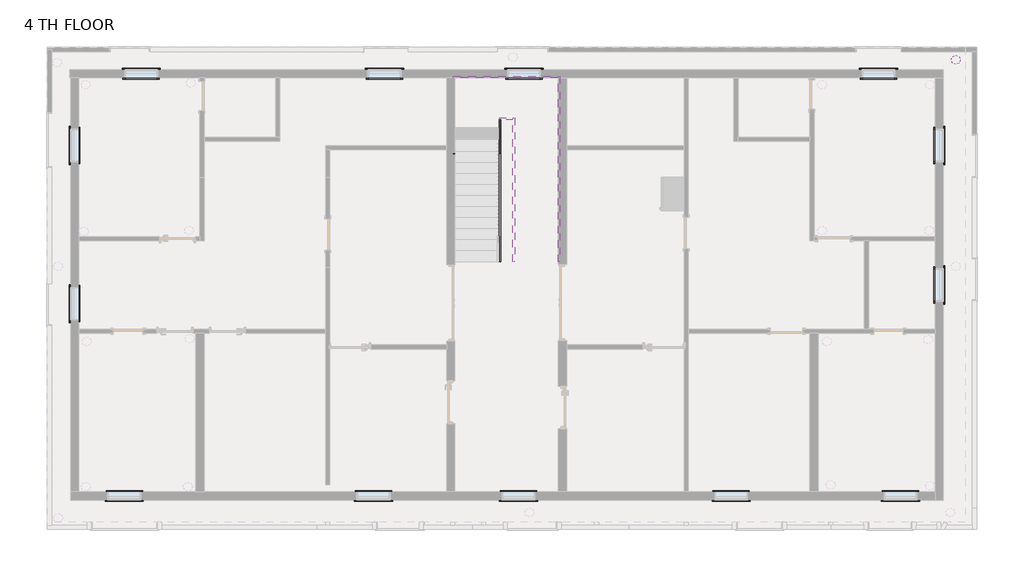
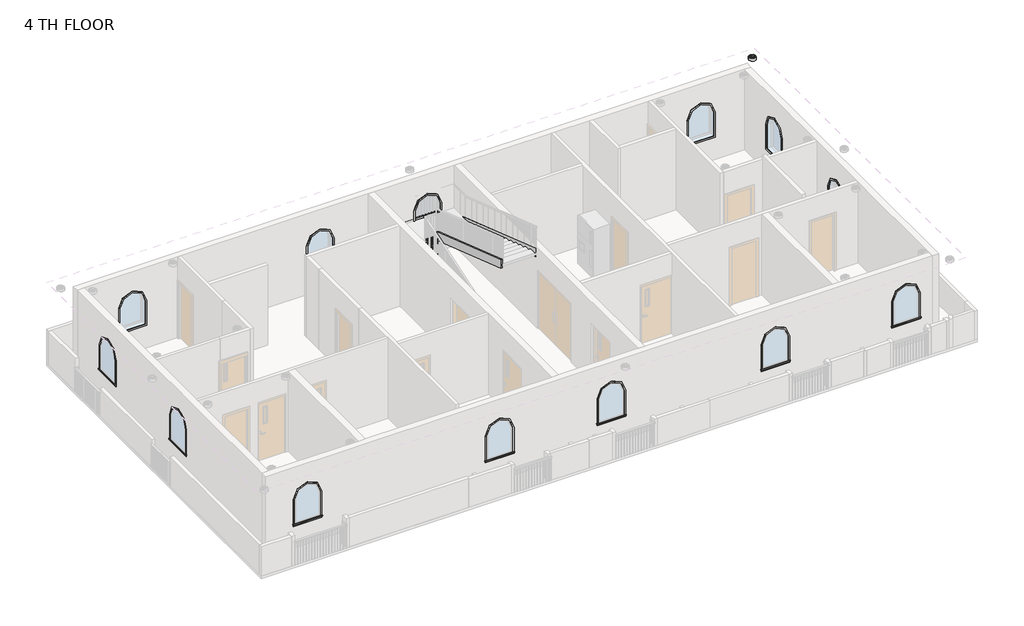
# One storey, part 7 of 7: 26 proxies, 6 members, 1 light fixture.
"""IFC4 building model written with IfcOpenShell, lengths in millimetres."""

from ifc_helpers import new_model, si_unit, frame, origin, place, context, project, spatial, polyline, outline, extrude, transform, mapped, element, save
from components import trim_window_exterior_flat_arch_top_tree_centered_with_sill_aed3e54d, trim_window_interior_flat_arch_top_tree_centered_picture_e2e46177, ceiling_light_flat_round_60w_120v_7c4c2a52

model = new_model("IFC4")

# Units and contexts
model_context = context("Model", 3, world=origin())
ifc_project = project(units=[si_unit("LENGTHUNIT", "METRE", prefix="MILLI")], contexts=[model_context])

# Site, building, storey
site = spatial("IfcSite", under=ifc_project)
building = spatial("IfcBuilding", under=site)
storey = spatial("IfcBuildingStorey", under=building, Name="4 TH FLOOR", Elevation=12801.6)

# Proxies
placement = place(None, origin())
trim_window_exterior_flat_arch_top_tree_centered_with_sill_shape = trim_window_exterior_flat_arch_top_tree_centered_with_sill_aed3e54d(model_context)
element("IfcBuildingElementProxy", 1, Name="Trim-Window-Exterior-Flat-Arch-Top-Tree_Centered : with Sill", ObjectType="Trim-Window-Exterior-Flat-Arch-Top-Tree_Centered : with Sill", at=placement, inside=storey, context=model_context, shape_type="MappedRepresentation", body=[
    mapped(trim_window_exterior_flat_arch_top_tree_centered_with_sill_shape, transform((-10967.3987925, -4014.0932193, 15087.6), x_axis=(1.0, 0.0, 0.0), y_axis=(0.0, 0.0, 1.0), z_axis=(0.0, -1.0, 0.0))),
])
element("IfcBuildingElementProxy", 2, Name="Trim-Window-Exterior-Flat-Arch-Top-Tree_Centered : with Sill", ObjectType="Trim-Window-Exterior-Flat-Arch-Top-Tree_Centered : with Sill", at=placement, inside=storey, context=model_context, shape_type="MappedRepresentation", body=[
    mapped(trim_window_exterior_flat_arch_top_tree_centered_with_sill_shape, transform((-4096.6987998, -4014.0932193, 15087.6), x_axis=(1.0, 0.0, 0.0), y_axis=(0.0, 0.0, 1.0), z_axis=(0.0, -1.0, 0.0))),
])
element("IfcBuildingElementProxy", 3, Name="Trim-Window-Exterior-Flat-Arch-Top-Tree_Centered : with Sill", ObjectType="Trim-Window-Exterior-Flat-Arch-Top-Tree_Centered : with Sill", at=placement, inside=storey, context=model_context, shape_type="MappedRepresentation", body=[
    mapped(trim_window_exterior_flat_arch_top_tree_centered_with_sill_shape, transform((-96.7067989, -4014.0932193, 15087.6), x_axis=(1.0, 0.0, 0.0), y_axis=(0.0, 0.0, 1.0), z_axis=(0.0, -1.0, 0.0))),
])
element("IfcBuildingElementProxy", 4, Name="Trim-Window-Exterior-Flat-Arch-Top-Tree_Centered : with Sill", ObjectType="Trim-Window-Exterior-Flat-Arch-Top-Tree_Centered : with Sill", at=placement, inside=storey, context=model_context, shape_type="MappedRepresentation", body=[
    mapped(trim_window_exterior_flat_arch_top_tree_centered_with_sill_shape, transform((5771.2012079, -4014.0932193, 15087.6), x_axis=(1.0, 0.0, 0.0), y_axis=(0.0, 0.0, 1.0), z_axis=(0.0, -1.0, 0.0))),
])
element("IfcBuildingElementProxy", 5, Name="Trim-Window-Exterior-Flat-Arch-Top-Tree_Centered : with Sill", ObjectType="Trim-Window-Exterior-Flat-Arch-Top-Tree_Centered : with Sill", at=placement, inside=storey, context=model_context, shape_type="MappedRepresentation", body=[
    mapped(trim_window_exterior_flat_arch_top_tree_centered_with_sill_shape, transform((10444.8012075, -4014.0932193, 15087.6), x_axis=(1.0, 0.0, 0.0), y_axis=(0.0, 0.0, 1.0), z_axis=(0.0, -1.0, 0.0))),
])
element("IfcBuildingElementProxy", 6, Name="Trim-Window-Exterior-Flat-Arch-Top-Tree_Centered : with Sill", ObjectType="Trim-Window-Exterior-Flat-Arch-Top-Tree_Centered : with Sill", at=placement, inside=storey, context=model_context, shape_type="MappedRepresentation", body=[
    mapped(trim_window_exterior_flat_arch_top_tree_centered_with_sill_shape, transform((11625.9012075, 1916.8067333, 15087.6), x_axis=(0.0, 1.0, 0.0), y_axis=(0.0, 0.0, 1.0), z_axis=(1.0, 0.0, 0.0))),
])
element("IfcBuildingElementProxy", 7, Name="Trim-Window-Exterior-Flat-Arch-Top-Tree_Centered : with Sill", ObjectType="Trim-Window-Exterior-Flat-Arch-Top-Tree_Centered : with Sill", at=placement, inside=storey, context=model_context, shape_type="MappedRepresentation", body=[
    mapped(trim_window_exterior_flat_arch_top_tree_centered_with_sill_shape, transform((11625.9012075, 5764.9067329, 15087.6), x_axis=(0.0, 1.0, 0.0), y_axis=(0.0, 0.0, 1.0), z_axis=(1.0, 0.0, 0.0))),
])
element("IfcBuildingElementProxy", 8, Name="Trim-Window-Exterior-Flat-Arch-Top-Tree_Centered : with Sill", ObjectType="Trim-Window-Exterior-Flat-Arch-Top-Tree_Centered : with Sill", at=placement, inside=storey, context=model_context, shape_type="MappedRepresentation", body=[
    mapped(trim_window_exterior_flat_arch_top_tree_centered_with_sill_shape, transform((9835.2012075, 7860.4067329, 15087.6), x_axis=(-1.0, 0.0, 0.0), y_axis=(0.0, 0.0, 1.0), z_axis=(0.0, 1.0, 0.0))),
])
element("IfcBuildingElementProxy", 9, Name="Trim-Window-Exterior-Flat-Arch-Top-Tree_Centered : with Sill", ObjectType="Trim-Window-Exterior-Flat-Arch-Top-Tree_Centered : with Sill", at=placement, inside=storey, context=model_context, shape_type="MappedRepresentation", body=[
    mapped(trim_window_exterior_flat_arch_top_tree_centered_with_sill_shape, transform((55.6932011, 7860.4067329, 15087.6), x_axis=(-1.0, 0.0, 0.0), y_axis=(0.0, 0.0, 1.0), z_axis=(0.0, 1.0, 0.0))),
])
element("IfcBuildingElementProxy", 10, Name="Trim-Window-Exterior-Flat-Arch-Top-Tree_Centered : with Sill", ObjectType="Trim-Window-Exterior-Flat-Arch-Top-Tree_Centered : with Sill", at=placement, inside=storey, context=model_context, shape_type="MappedRepresentation", body=[
    mapped(trim_window_exterior_flat_arch_top_tree_centered_with_sill_shape, transform((-3791.8987998, 7860.4067329, 15087.6), x_axis=(-1.0, 0.0, 0.0), y_axis=(0.0, 0.0, 1.0), z_axis=(0.0, 1.0, 0.0))),
])
element("IfcBuildingElementProxy", 11, Name="Trim-Window-Exterior-Flat-Arch-Top-Tree_Centered : with Sill", ObjectType="Trim-Window-Exterior-Flat-Arch-Top-Tree_Centered : with Sill", at=placement, inside=storey, context=model_context, shape_type="MappedRepresentation", body=[
    mapped(trim_window_exterior_flat_arch_top_tree_centered_with_sill_shape, transform((-10503.8487992, 7860.4067329, 15087.6), x_axis=(-1.0, 0.0, 0.0), y_axis=(0.0, 0.0, 1.0), z_axis=(0.0, 1.0, 0.0))),
])
element("IfcBuildingElementProxy", 12, Name="Trim-Window-Exterior-Flat-Arch-Top-Tree_Centered : with Sill", ObjectType="Trim-Window-Exterior-Flat-Arch-Top-Tree_Centered : with Sill", at=placement, inside=storey, context=model_context, shape_type="MappedRepresentation", body=[
    mapped(trim_window_exterior_flat_arch_top_tree_centered_with_sill_shape, transform((-12453.2987925, 5764.9067329, 15087.6), x_axis=(0.0, -1.0, 0.0), y_axis=(0.0, 0.0, 1.0), z_axis=(-1.0, 0.0, 0.0))),
])
element("IfcBuildingElementProxy", 13, Name="Trim-Window-Exterior-Flat-Arch-Top-Tree_Centered : with Sill", ObjectType="Trim-Window-Exterior-Flat-Arch-Top-Tree_Centered : with Sill", at=placement, inside=storey, context=model_context, shape_type="MappedRepresentation", body=[
    mapped(trim_window_exterior_flat_arch_top_tree_centered_with_sill_shape, transform((-12453.2987925, 1402.4567334, 15087.6), x_axis=(0.0, -1.0, 0.0), y_axis=(0.0, 0.0, 1.0), z_axis=(-1.0, 0.0, 0.0))),
])
trim_window_interior_flat_arch_top_tree_centered_picture_shape = trim_window_interior_flat_arch_top_tree_centered_picture_e2e46177(model_context)
element("IfcBuildingElementProxy", 14, Name="Trim-Window-Interior-Flat-Arch-Top-Tree_Centered : Picture Frame", ObjectType="Trim-Window-Interior-Flat-Arch-Top-Tree_Centered : Picture Frame", at=placement, inside=storey, context=model_context, shape_type="MappedRepresentation", body=[
    mapped(trim_window_interior_flat_arch_top_tree_centered_picture_shape, transform((-10967.3987925, -3785.4932193, 15087.6), x_axis=(-1.0, 0.0, 0.0), y_axis=(0.0, 0.0, 1.0), z_axis=(0.0, 1.0, 0.0))),
])
element("IfcBuildingElementProxy", 15, Name="Trim-Window-Interior-Flat-Arch-Top-Tree_Centered : Picture Frame", ObjectType="Trim-Window-Interior-Flat-Arch-Top-Tree_Centered : Picture Frame", at=placement, inside=storey, context=model_context, shape_type="MappedRepresentation", body=[
    mapped(trim_window_interior_flat_arch_top_tree_centered_picture_shape, transform((-4096.6987998, -3785.4932193, 15087.6), x_axis=(-1.0, 0.0, 0.0), y_axis=(0.0, 0.0, 1.0), z_axis=(0.0, 1.0, 0.0))),
])
element("IfcBuildingElementProxy", 16, Name="Trim-Window-Interior-Flat-Arch-Top-Tree_Centered : Picture Frame", ObjectType="Trim-Window-Interior-Flat-Arch-Top-Tree_Centered : Picture Frame", at=placement, inside=storey, context=model_context, shape_type="MappedRepresentation", body=[
    mapped(trim_window_interior_flat_arch_top_tree_centered_picture_shape, transform((-96.7067989, -3785.4932193, 15087.6), x_axis=(-1.0, 0.0, 0.0), y_axis=(0.0, 0.0, 1.0), z_axis=(0.0, 1.0, 0.0))),
])
element("IfcBuildingElementProxy", 17, Name="Trim-Window-Interior-Flat-Arch-Top-Tree_Centered : Picture Frame", ObjectType="Trim-Window-Interior-Flat-Arch-Top-Tree_Centered : Picture Frame", at=placement, inside=storey, context=model_context, shape_type="MappedRepresentation", body=[
    mapped(trim_window_interior_flat_arch_top_tree_centered_picture_shape, transform((5771.2012079, -3785.4932193, 15087.6), x_axis=(-1.0, 0.0, 0.0), y_axis=(0.0, 0.0, 1.0), z_axis=(0.0, 1.0, 0.0))),
])
element("IfcBuildingElementProxy", 18, Name="Trim-Window-Interior-Flat-Arch-Top-Tree_Centered : Picture Frame", ObjectType="Trim-Window-Interior-Flat-Arch-Top-Tree_Centered : Picture Frame", at=placement, inside=storey, context=model_context, shape_type="MappedRepresentation", body=[
    mapped(trim_window_interior_flat_arch_top_tree_centered_picture_shape, transform((10444.8012075, -3785.4932193, 15087.6), x_axis=(-1.0, 0.0, 0.0), y_axis=(0.0, 0.0, 1.0), z_axis=(0.0, 1.0, 0.0))),
])
element("IfcBuildingElementProxy", 19, Name="Trim-Window-Interior-Flat-Arch-Top-Tree_Centered : Picture Frame", ObjectType="Trim-Window-Interior-Flat-Arch-Top-Tree_Centered : Picture Frame", at=placement, inside=storey, context=model_context, shape_type="MappedRepresentation", body=[
    mapped(trim_window_interior_flat_arch_top_tree_centered_picture_shape, transform((11397.3012075, 1916.8067333, 15087.6), x_axis=(0.0, -1.0, 0.0), y_axis=(0.0, 0.0, 1.0), z_axis=(-1.0, 0.0, 0.0))),
])
element("IfcBuildingElementProxy", 20, Name="Trim-Window-Interior-Flat-Arch-Top-Tree_Centered : Picture Frame", ObjectType="Trim-Window-Interior-Flat-Arch-Top-Tree_Centered : Picture Frame", at=placement, inside=storey, context=model_context, shape_type="MappedRepresentation", body=[
    mapped(trim_window_interior_flat_arch_top_tree_centered_picture_shape, transform((11397.3012075, 5764.9067329, 15087.6), x_axis=(0.0, -1.0, 0.0), y_axis=(0.0, 0.0, 1.0), z_axis=(-1.0, 0.0, 0.0))),
])
element("IfcBuildingElementProxy", 21, Name="Trim-Window-Interior-Flat-Arch-Top-Tree_Centered : Picture Frame", ObjectType="Trim-Window-Interior-Flat-Arch-Top-Tree_Centered : Picture Frame", at=placement, inside=storey, context=model_context, shape_type="MappedRepresentation", body=[
    mapped(trim_window_interior_flat_arch_top_tree_centered_picture_shape, transform((9835.2012075, 7631.8067329, 15087.6), x_axis=(1.0, 0.0, 0.0), y_axis=(0.0, 0.0, 1.0), z_axis=(0.0, -1.0, 0.0))),
])
element("IfcBuildingElementProxy", 22, Name="Trim-Window-Interior-Flat-Arch-Top-Tree_Centered : Picture Frame", ObjectType="Trim-Window-Interior-Flat-Arch-Top-Tree_Centered : Picture Frame", at=placement, inside=storey, context=model_context, shape_type="MappedRepresentation", body=[
    mapped(trim_window_interior_flat_arch_top_tree_centered_picture_shape, transform((55.6932011, 7631.8067329, 15087.6), x_axis=(1.0, 0.0, 0.0), y_axis=(0.0, 0.0, 1.0), z_axis=(0.0, -1.0, 0.0))),
])
element("IfcBuildingElementProxy", 23, Name="Trim-Window-Interior-Flat-Arch-Top-Tree_Centered : Picture Frame", ObjectType="Trim-Window-Interior-Flat-Arch-Top-Tree_Centered : Picture Frame", at=placement, inside=storey, context=model_context, shape_type="MappedRepresentation", body=[
    mapped(trim_window_interior_flat_arch_top_tree_centered_picture_shape, transform((-3791.8987998, 7631.8067329, 15087.6), x_axis=(1.0, 0.0, 0.0), y_axis=(0.0, 0.0, 1.0), z_axis=(0.0, -1.0, 0.0))),
])
element("IfcBuildingElementProxy", 24, Name="Trim-Window-Interior-Flat-Arch-Top-Tree_Centered : Picture Frame", ObjectType="Trim-Window-Interior-Flat-Arch-Top-Tree_Centered : Picture Frame", at=placement, inside=storey, context=model_context, shape_type="MappedRepresentation", body=[
    mapped(trim_window_interior_flat_arch_top_tree_centered_picture_shape, transform((-10503.8487992, 7631.8067329, 15087.6), x_axis=(1.0, 0.0, 0.0), y_axis=(0.0, 0.0, 1.0), z_axis=(0.0, -1.0, 0.0))),
])
element("IfcBuildingElementProxy", 25, Name="Trim-Window-Interior-Flat-Arch-Top-Tree_Centered : Picture Frame", ObjectType="Trim-Window-Interior-Flat-Arch-Top-Tree_Centered : Picture Frame", at=placement, inside=storey, context=model_context, shape_type="MappedRepresentation", body=[
    mapped(trim_window_interior_flat_arch_top_tree_centered_picture_shape, transform((-12224.6987925, 5764.9067329, 15087.6), x_axis=(0.0, 1.0, 0.0), y_axis=(0.0, 0.0, 1.0), z_axis=(1.0, 0.0, 0.0))),
])
element("IfcBuildingElementProxy", 26, Name="Trim-Window-Interior-Flat-Arch-Top-Tree_Centered : Picture Frame", ObjectType="Trim-Window-Interior-Flat-Arch-Top-Tree_Centered : Picture Frame", at=placement, inside=storey, context=model_context, shape_type="MappedRepresentation", body=[
    mapped(trim_window_interior_flat_arch_top_tree_centered_picture_shape, transform((-12224.6987925, 1402.4567334, 15087.6), x_axis=(0.0, 1.0, 0.0), y_axis=(0.0, 0.0, 1.0), z_axis=(1.0, 0.0, 0.0))),
])

# Light fixture
ceiling_light_flat_round_60w_120v_shape = ceiling_light_flat_round_60w_120v_7c4c2a52(model_context)
element("IfcLightFixture", 27, ObjectType="Ceiling Light - Flat Round : 60W - 120V", at=placement, inside=storey, context=model_context, shape_type="MappedRepresentation", body=[
    mapped(ceiling_light_flat_round_60w_120v_shape, transform((11968.8012075, 8127.1067329, 13411.2), x_axis=(1.0, 0.0, 0.0), y_axis=(0.0, 1.0, 0.0), z_axis=(0.0, 0.0, 1.0))),
])

# Members
element("IfcMember", 28, ObjectType="Stringer - 2\" Width", at=placement, inside=storey, context=model_context, shape_type="SweptSolid", body=[
    extrude(outline(polyline([(2564.5067329, 12801.6), (2564.5067329, 12994.838056), (6486.7524627, 14325.6), (7435.4093802, 14325.6), (2943.6199065, 12801.6), (2564.5067329, 12801.6)])), frame((-1899.5987998, 0.0, 0.0), z_axis=(1.0, 0.0, 0.0), x_axis=(0.0, 1.0, 0.0)), (0.0, 0.0, 1.0), 50.8),
])
element("IfcMember", 29, ObjectType="Stringer - 2\" Width", at=placement, inside=storey, context=model_context, shape_type="SweptSolid", body=[
    extrude(outline(polyline([(-1899.5987998, 7631.8067329), (-1899.5987998, 7682.6067329), (996.0012002, 7682.6067329), (996.0012002, 7631.8067329), (-1899.5987998, 7631.8067329)])), frame((0.0, 0.0, 14020.8), z_axis=(0.0, 0.0, 1.0), x_axis=(1.0, 0.0, 0.0)), (0.0, 0.0, 1.0), 304.8),
])
element("IfcMember", 30, ObjectType="Stringer - 2\" Width", at=placement, inside=storey, context=model_context, shape_type="SweptSolid", body=[
    extrude(outline(polyline([(7682.6067329, 14050.525556), (7682.6067329, 14020.8), (6821.5619804, 14020.8), (2564.5067329, 15465.1580304), (2564.5067329, 15787.0237702), (7682.6067329, 14050.525556)])), frame((996.0012002, 0.0, 0.0), z_axis=(1.0, 0.0, 0.0), x_axis=(0.0, 1.0, 0.0)), (0.0, 0.0, 1.0), 50.8),
])
element("IfcMember", 31, ObjectType="Stringer - 2\" Width", at=placement, inside=storey, context=model_context, shape_type="SweptSolid", body=[
    extrude(outline(polyline([(2564.5067329, 12801.6), (2564.5067329, 12994.838056), (6476.1067329, 14321.988056), (6476.1067329, 14000.1223161), (2943.6199065, 12801.6), (2564.5067329, 12801.6)])), frame((-629.5987998, 0.0, 0.0), z_axis=(1.0, 0.0, 0.0), x_axis=(0.0, 1.0, 0.0)), (0.0, 0.0, 1.0), 50.8),
])
element("IfcMember", 32, ObjectType="Stringer - 2\" Width", at=placement, inside=storey, context=model_context, shape_type="SweptSolid", body=[
    extrude(outline(polyline([(-629.5987998, 6476.1067329), (-629.5987998, 6526.9067329), (-248.5987915, 6526.9067329), (-248.5987915, 6476.1067329), (-629.5987998, 6476.1067329)])), frame((0.0, 0.0, 14020.8), z_axis=(0.0, 0.0, 1.0), x_axis=(1.0, 0.0, 0.0)), (0.0, 0.0, 1.0), 304.8),
])
element("IfcMember", 33, ObjectType="Stringer - 2\" Width", at=placement, inside=storey, context=model_context, shape_type="SweptSolid", body=[
    extrude(outline(polyline([(6526.9067329, 14442.638056), (6526.9067329, 14120.7723161), (2564.5067329, 15465.1580304), (2564.5067329, 15787.0237702), (6526.9067329, 14442.638056)])), frame((-248.5987915, 0.0, 0.0), z_axis=(1.0, 0.0, 0.0), x_axis=(0.0, 1.0, 0.0)), (0.0, 0.0, 1.0), 50.8),
])

save(model, "model.ifc")

# Revit data of these elements
# Type "Trim-Window-Exterior-Flat-Arch-Top-Tree_Centered : with Sill"
#   Trim Width = 0' - 2 1/4"
#   Trim Thickness_Picture Frame = 0' - 1 1/4"
#   Trim Thickness_with Sill = 0' - 0 3/4"
#   Sill Thickness = 0' - 1 1/4"
#   Opening Width [instance default] = 2' - 0"
#   Opening Height [instance default] = 3' - 0"
#   Default Elevation = 4' - 0"
#   Sill = yes
#   Picture Frame = no
#   Trim Material [instance default] = none
# Type "Trim-Window-Interior-Flat-Arch-Top-Tree_Centered : Picture Frame"
#   Trim Thickness_Picture Frame = 0' - 1 1/4"
#   Trim Width = 0' - 2 1/4"
#   Trim Thickness_with Sill = 0' - 0 3/4"
#   Sill Thickness = 0' - 1 1/4"
#   Opening Width [instance default] = 2' - 0"
#   Opening Height [instance default] = 3' - 0"
#   Default Elevation = 4' - 0"
#   Sill = no
#   Picture Frame = yes
#   Trim Material [instance default] = none
# Type "Ceiling Light - Flat Round : 60W - 120V"
#   Lamp = "A-19"
#   Assembly Code = "D5020220"
#   Wattage = 60 W
#   built-in parameter 1150110 = 1 (stored number, unit not read)
#   built-in parameter 1114217 = 1 (stored number, unit not read)
#   built-in parameter 1150109 = 1 (stored number, unit not read)
#   built-in parameter 1150113 = 1 (stored number, unit not read)
#   built-in parameter 1150115 = 1 (stored number, unit not read)
#   built-in parameter 1150105 = 272.155 (stored number, unit not read)
#   Light Source Symbol Size = 2' - 0"
#   built-in parameter 1150112 = 1 (stored number, unit not read)
#   built-in parameter 1150114 = 1 (stored number, unit not read)
#   built-in parameter 1150107 = 2800 (stored number, unit not read)
#   built-in parameter 1150106 = 2.72155 (stored number, unit not read)
#   Emit from Circle Diameter = 0' - 10"
#   built-in parameter 1150104 = 1.32387 (stored number, unit not read)
#   Ballast Voltage = 120 V
#   built-in parameter 1114218 = 1 (stored number, unit not read)
#   built-in parameter 1150133 = 10 (stored number, unit not read)
#   Lumens = 855 lm
#   Apparent Load = 60 VA
#   built-in parameter 1150134 = 4
#   built-in parameter 1150137 = 1
#   Color Filter = 16777215
#   built-in parameter 1140040 [instance default] = 1
#   Ballast Number of Poles = 1
#   Light Box Material = Steel, Paint Finish, Dark Gray, Matte
#   Diffuser Material = Glass, White, High Luminance
#   Wattage Comments = ""
#   Emit Shape Visible in Rendering = no
#   Dimming Lamp Color Temperature Shift = (empty or 0)
#   Default Elevation = 0
# Elements 1, 2, 3, 4, 5, 6, 7, 8, 9, 10, 11, 12, 13 (IfcBuildingElementProxy, "Trim-Window-Exterior-Flat-Arch-Top-Tree_Centered : with Sill")
#   Opening Width = 3' - 0"
#   Opening Height = 4' - 6"
#   Trim Material = Clad - White
#   Phase Created = New Construction
#   Materials on its faces: "Clad - White"
# Elements 14, 15, 16, 17, 18, 19, 20, 21, 22, 23, 24, 25, 26 (IfcBuildingElementProxy, "Trim-Window-Interior-Flat-Arch-Top-Tree_Centered : Picture Frame")
#   Opening Width = 3' - 0"
#   Opening Height = 4' - 6"
#   Trim Material = Wood - Stained
#   Phase Created = New Construction
#   Materials on its faces: "Wood - Stained"
# Element 27 (IfcLightFixture, "Ceiling Light - Flat Round : 60W - 120V")
#   Mark = "114"
#   built-in parameter 1140040 = 1
#   Phase Created = New Construction
#   Materials on its faces: "Glass, White, High Luminance", "Steel, Paint Finish, Dark Gray, Matte"
# Elements 28, 29, 30, 31, 32, 33 (IfcMember, "Stringer - 2\" Width")
#   Phase Created = New Construction
# Materials
#   "Steel, Paint Finish, Dark Gray, Matte": class "Metal", colour RGB 98 98 98, transparency 0, Description = "Steel, paint finish, dark gray, matte", Cost = 0
#   "Glass, White, High Luminance": class "Glass", colour RGB 249 250 249, transparency 0.8, Description = "physical material", Cost = 0
#   "Clad - White": class "Wood", colour RGB 242 242 238, transparency 0, Cost = 0
#   "Wood - Stained": class "Wood", colour RGB 224 178 126, transparency 0, Cost = 0
